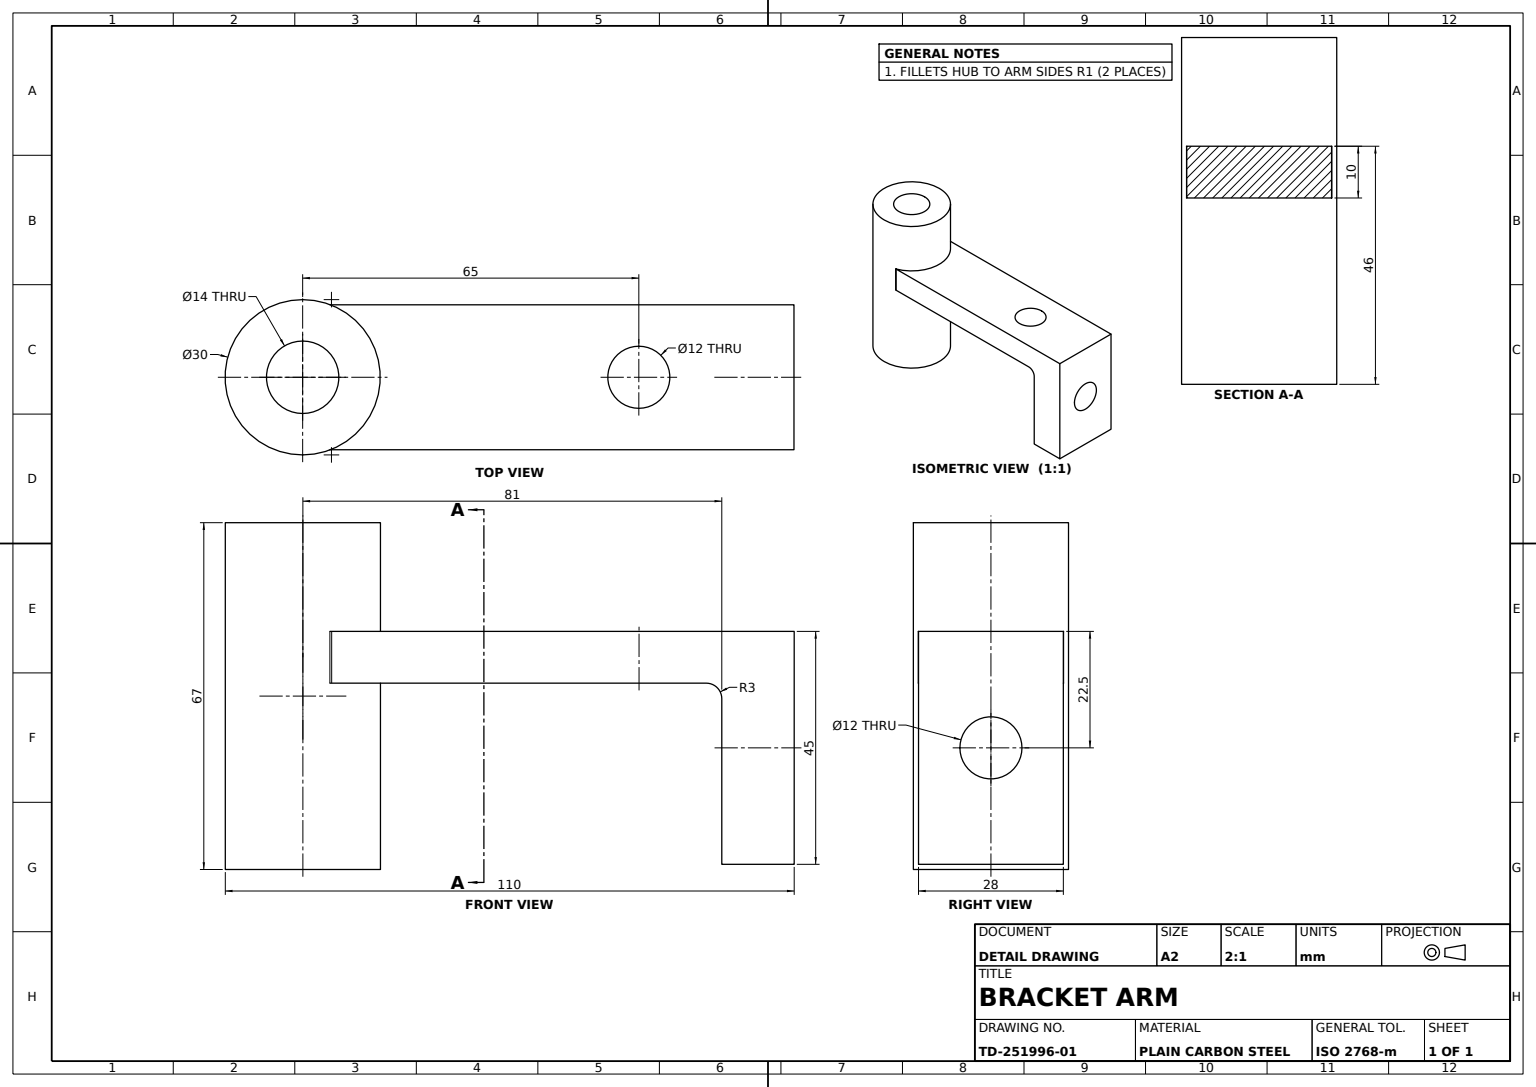
SolidWorks part; units mm, degrees
material "Plain Carbon Steel"
ref_plane "Front Plane" through (0, 0, 0) normal (0, 0, 1) x (1, 0, 0)
ref_plane "Top Plane" through (0, 0, 0) normal (0, 1, 0) x (1, 0, 0)
ref_plane "Right Plane" through (0, 0, 0) normal (1, 0, 0) x (0, 0, -1)
sketch "Arm Profile Sketch" plane through (0, 0, 0) normal (0, 0, 1) x (1, 0, 0)
  line L0 (0, 0) -> (78, 0)
  line L1 (81, -3) -> (81, -35)
  line L2 (81, -35) -> (95, -35)
  line L3 (95, -35) -> (95, 10)
  line L4 (95, 10) -> (0, 10)
  line L5 (0, 10) -> (0, 0)
  arc A0 (78, 0) -> (81, -3) centre (78, -3) cw
  dimension "D1" = 3
  dimension "D2" = 81
  dimension "D3" = 95
  dimension "D4" = 35
  dimension "D5" = 45
extrude "Crank Arm" add sketch "Arm Profile Sketch" along normal blind 28
sketch "Pivot Hub Sketch" plane through (0, 10, 0) normal (0, 1, 0) x (1, 0, 0)
  line L0 (0, -28) -> (0, 0) construction
  circle A0 centre (0, -14) radius 15
  circle A1 centre (0, -14) radius 7
  dimension "D1" = 14
  dimension "D2" = 30
extrude "Pivot Hub" add sketch "Pivot Hub Sketch" against normal blind 46 and the other way blind 21
fillet "Hub Fillet R1" radius 1 2 edges at (5.3852, 5, 0) (5.3852, 5, 28)
sketch "Top Hole Sketch" plane through (0, 0, 0) normal (0, 1, 0) x (1, 0, 0)
  line L1 (0, -7) -> (0, -21)
  line L2 (0, -7) -> (0, -21)
  arc A1 (0, -21) -> (0, -7) centre (0, -14) ccw
  arc A2 (0, -21) -> (0, -7) centre (0, -14) ccw
  dimension "D1" = 0
extrude "Top Through Hole" cut sketch "Top Hole Sketch" along normal blind 132
sketch "Arm Hole Sketch" plane through (0, 10, 0) normal (0, 1, 0) x (1, 0, 0)
  line L0 (95, -14) -> (65, -14) construction
  line L1 (95, -28) -> (95, 0) construction
  circle A0 centre (65, -14) radius 6
  dimension "D1" = 12
  dimension "D2" = 30
extrude "Arm Through Hole" cut sketch "Arm Hole Sketch" against normal blind 132
sketch "Bore Sketch" plane through (95, 0, 0) normal (1, 0, 0) x (0, 0, -1)
  line L0 (0, -35) -> (0, 10) construction
  line L1 (-28, 10) -> (0, 10) construction
  circle A0 centre (-14, -12.5) radius 6
  dimension "D1" = 12
  dimension "D2" = 14
  dimension "D3" = 22.5
extrude "Through Bore" cut sketch "Bore Sketch" against normal blind 42
